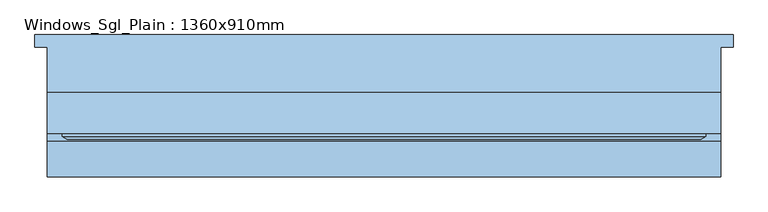
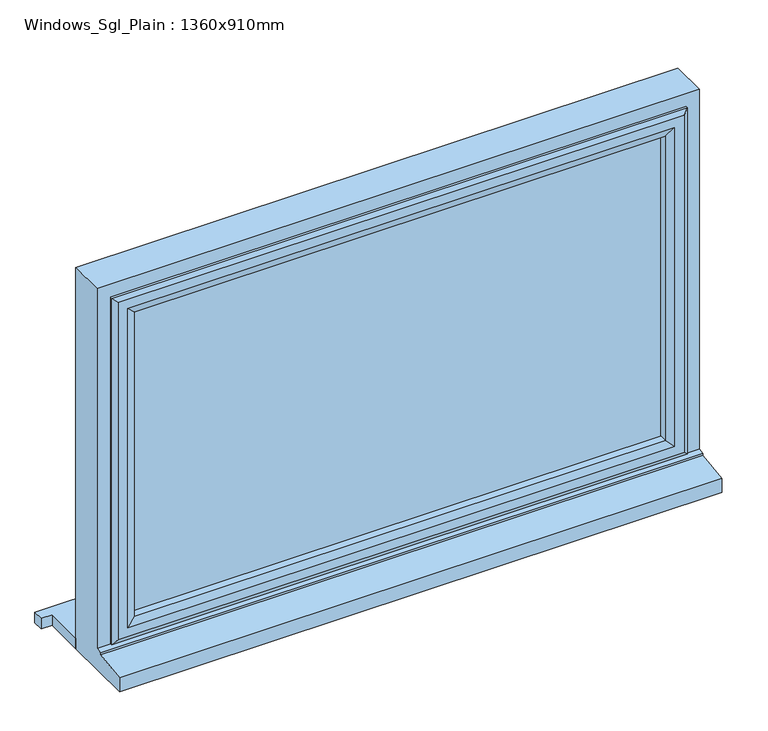
"""IFC4 building model written with IfcOpenShell, lengths in millimetres: window geometry, Windows_Sgl_Plain : 1360x910mm."""

from ifc_helpers import new_model, si_unit, frame, origin, place, context, project, spatial, polyline, outline, extrude, faceted_brep, source, transform, mapped, element, save


def windows_sgl_plain_1360x910mm_8a2bb76a(model_context):
    return source(origin(), model_context, "Body", "SolidModel", [
        extrude(outline(polyline([(-705.0, 129.0434322), (705.0, 129.0434322), (705.0, 104.0434322), (680.0, 104.0434322), (680.0, 12.0434322), (-680.0, 12.0434322), (-680.0, 104.0434322), (-705.0, 104.0434322), (-705.0, 129.0434322)])), frame((0.0, 0.0, 1200.0), z_axis=(0.0, 0.0, 1.0), x_axis=(1.0, 0.0, 0.0)), (0.0, 0.0, 1.0), 25.0),
        faceted_brep([(-680.0, 12.0434322, 1200.0), (-680.0, 12.0434322, 2110.0), (680.0, 12.0434322, 2110.0), (680.0, 12.0434322, 1200.0), (-620.0, 12.0434322, 2050.0), (-620.0, 12.0434322, 1275.0), (620.0, 12.0434322, 1275.0), (620.0, 12.0434322, 2050.0), (-680.0, -158.4565678, 1200.0), (-680.0, -158.4565678, 1233.8088847), (-680.0, -85.9565678, 1244.7449676), (-680.0, -85.9565678, 1249.68767), (-680.0, -70.9565678, 1251.0), (-680.0, -70.9565678, 2110.0), (680.0, -70.9565678, 1251.0), (680.0, -70.9565678, 2110.0), (-640.0, -70.9565678, 2070.0), (640.0, -70.9565678, 2070.0), (640.0, -70.9565678, 1263.0), (-640.0, -70.9565678, 1263.0), (-640.0, -5.9565678, 1263.0), (-640.0, -5.9565678, 2070.0), (640.0, -5.9565678, 1263.0), (640.0, -5.9565678, 2070.0), (-620.0, -5.9565678, 2050.0), (620.0, -5.9565678, 2050.0), (620.0, -5.9565678, 1275.0), (-620.0, -5.9565678, 1275.0), (680.0, -85.9565678, 1249.68767), (680.0, -85.9565678, 1244.7449676), (680.0, -158.4565678, 1233.8088847), (680.0, -158.4565678, 1200.0)], [[[0, 1, 2, 3], [4, 5, 6, 7]], [[0, 8, 9, 10, 11, 12, 13, 1]], [[12, 14, 15, 13], [16, 17, 18, 19]], [[19, 20, 21, 16]], [[21, 20, 22, 23], [24, 25, 26, 27]], [[24, 27, 5, 4]], [[1, 13, 15, 2]], [[16, 21, 23, 17]], [[7, 25, 24, 4]], [[14, 28, 29, 30, 31, 3, 2, 15]], [[17, 23, 22, 18]], [[7, 6, 26, 25]], [[31, 8, 0, 3]], [[30, 9, 8, 31]], [[29, 10, 9, 30]], [[28, 11, 10, 29]], [[14, 12, 11, 28]], [[20, 19, 18, 22]], [[5, 27, 26, 6]]]),
        extrude(outline(polyline([(610.0, -34.9565678), (610.0, -58.9565678), (-610.0, -58.9565678), (-610.0, -34.9565678), (610.0, -34.9565678)])), frame((0.0, 0.0, 1293.0), z_axis=(0.0, 0.0, 1.0), x_axis=(1.0, 0.0, 0.0)), (0.0, 0.0, 1.0), 747.0),
        faceted_brep([(-650.0, -70.9565678, 2080.0), (-650.0, -70.9565678, 1253.0), (-650.0, -76.7300705, 1253.0), (-650.0, -76.7300705, 2080.0), (-640.0, -5.9565678, 2070.0), (-640.0, -5.9565678, 1263.0), (-640.0, -70.9565678, 1263.0), (-640.0, -70.9565678, 2070.0), (-600.0, -20.4494677, 2030.0), (-600.0, -20.4494677, 1303.0), (-610.1480377, -5.9565678, 1292.8519623), (-610.1480377, -5.9565678, 2040.1480377), (-600.0, -34.9565678, 2030.0), (-600.0, -34.9565678, 1303.0), (-610.0, -58.9565678, 2040.0), (-610.0, -58.9565678, 1293.0), (-610.0, -34.9565678, 1293.0), (-610.0, -34.9565678, 2040.0), (-600.0, -76.7300705, 2030.0), (-600.0, -76.7300705, 1303.0), (-600.0, -58.9565678, 1303.0), (-600.0, -58.9565678, 2030.0), (-617.4457548, -82.5035732, 2047.4457548), (-617.4457548, -82.5035732, 1285.5542452), (-639.2153903, -82.5035732, 1263.7846097), (-639.2153903, -82.5035732, 2069.2153903), (650.0, -70.9565678, 1253.0), (650.0, -76.7300705, 1253.0), (640.0, -5.9565678, 1263.0), (640.0, -70.9565678, 1263.0), (600.0, -20.4494677, 1303.0), (610.1480377, -5.9565678, 1292.8519623), (600.0, -34.9565678, 1303.0), (610.0, -58.9565678, 1293.0), (610.0, -34.9565678, 1293.0), (600.0, -76.7300705, 1303.0), (600.0, -58.9565678, 1303.0), (617.4457548, -82.5035732, 1285.5542452), (639.2153903, -82.5035732, 1263.7846097), (650.0, -70.9565678, 2080.0), (650.0, -76.7300705, 2080.0), (640.0, -5.9565678, 2070.0), (640.0, -70.9565678, 2070.0), (600.0, -20.4494677, 2030.0), (610.1480377, -5.9565678, 2040.1480377), (600.0, -34.9565678, 2030.0), (610.0, -58.9565678, 2040.0), (610.0, -34.9565678, 2040.0), (600.0, -76.7300705, 2030.0), (600.0, -58.9565678, 2030.0), (617.4457548, -82.5035732, 2047.4457548), (639.2153903, -82.5035732, 2069.2153903)], [[[0, 1, 2, 3]], [[4, 5, 6, 7]], [[8, 9, 10, 11]], [[12, 13, 9, 8]], [[14, 15, 16, 17]], [[18, 19, 20, 21]], [[22, 23, 19, 18]], [[3, 2, 24, 25]], [[1, 26, 27, 2]], [[5, 28, 29, 6]], [[9, 30, 31, 10]], [[13, 32, 30, 9]], [[15, 33, 34, 16]], [[19, 35, 36, 20]], [[23, 37, 35, 19]], [[2, 27, 38, 24]], [[26, 39, 40, 27]], [[28, 41, 42, 29]], [[30, 43, 44, 31]], [[32, 45, 43, 30]], [[33, 46, 47, 34]], [[35, 48, 49, 36]], [[37, 50, 48, 35]], [[27, 40, 51, 38]], [[39, 0, 3, 40]], [[1, 0, 39, 26], [7, 6, 29, 42]], [[41, 4, 7, 42]], [[5, 4, 41, 28], [11, 10, 31, 44]], [[43, 8, 11, 44]], [[45, 12, 8, 43]], [[17, 16, 34, 47], [13, 12, 45, 32]], [[46, 14, 17, 47]], [[15, 14, 46, 33], [21, 20, 36, 49]], [[48, 18, 21, 49]], [[50, 22, 18, 48]], [[25, 24, 38, 51], [23, 22, 50, 37]], [[40, 3, 25, 51]]]),
    ])


if __name__ == "__main__":
    model = new_model("IFC4")
    model_context = context("Model", 3, world=origin())
    ifc_project = project(units=[si_unit("LENGTHUNIT", "METRE", prefix="MILLI")], contexts=[model_context])
    site = spatial("IfcSite", under=ifc_project)
    building = spatial("IfcBuilding", under=site)
    placement = place(None, origin())
    windows_sgl_plain_1360x910mm_shape = windows_sgl_plain_1360x910mm_8a2bb76a(model_context)
    element("IfcWindow", 1, ObjectType="Windows_Sgl_Plain : 1360x910mm", at=placement, inside=building, context=model_context, shape_type="MappedRepresentation", body=[
        mapped(windows_sgl_plain_1360x910mm_shape, transform((0.0, 0.0, 0.0), x_axis=(1.0, 0.0, 0.0), y_axis=(0.0, 1.0, 0.0), z_axis=(0.0, 0.0, 1.0))),
    ])
    save(model, "model.ifc")

# Revit data of these elements
# Type "Windows_Sgl_Plain : 1360x910mm"
#   Type Mark = "46"
#   Operation = "SinglePanel"
#   Construction Type Id = "SGL"
#   Manufacturer = "Revit"
#   Keynote = "L10"
#   Analytic Construction = "Large single-glazed windows"
#   Wrap Layers (Ext) from Ext = 102.5 mm
#   Wrap Layers (Int) from Ext = 177.5 mm
#   Window Board Projection = 25 mm
#   Window Board Extension = 25 mm
#   Visual Light Transmittance = 0.9
#   Solar Heat Gain Coefficient = 0.86
#   Rough Width = 1360 mm
#   Rough Height = 910 mm
#   Height = 910 mm
#   Width = 1360 mm
#   Heat Transfer Coefficient (U) = 5.5617 W/(m²·K)
#   Glazing Thickness = 24 mm
#   FrameOffset - External = 50 mm
#   Frame Depth = 65 mm
#   Default Head Height = 2110 mm
#   Cill Depth = 87.5 mm
#   Cavity Closer Width = 50 mm
#   Cavity Closer Offset from Ext = 102.5 mm
#   Cavity Closer Depth = 85 mm
#   Define Thermal Properties by = 1
#   Vis - Cavity Closers = yes
#   Define Thermal Properties by = 1
#   Material Trim = Window Frame
#   Material Glass = Glass
#   Material Frame = Window Frame
#   Wall Closure = (empty or 0)
# Element 1 (IfcWindow, "Windows_Sgl_Plain : 1360x910mm")
#   Materials on its faces: "Window Frame", "Glass"
# Materials
#   "Window Frame": colour RGB 249 249 249, transparency 0, Keynote = "L10", Cost = 0
#   "Glass": class "Glass", colour RGB 0 128 192, transparency 0.9, Description = "Soda Lime Glass", Cost = 0
